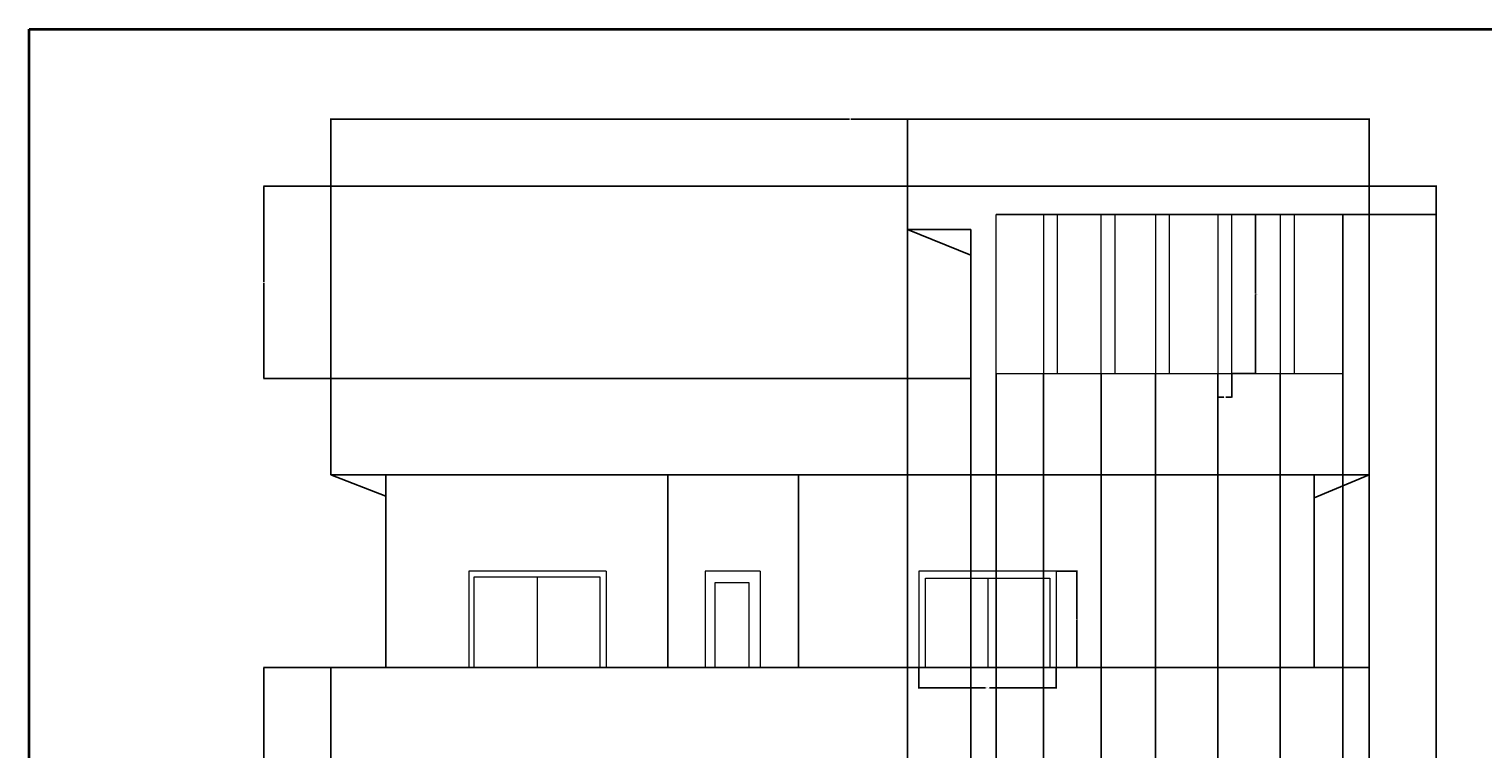
# Model space of a CAD drawing. Units: inches. Extents: x 1955 to 3324, y 980 to 3129.
# Tile 10 of 11: x 1955 to 2589, y 2815 to 3129. Entities that reach past the tile are written whole.
import ezdxf

# ---------------------------------------------------------------- set-up
doc = ezdxf.new("R2010")
doc.units = ezdxf.units.IN
for name, color, linetype, lineweight in [('A-ANNO-DIMS', 2, 'Continuous', 18), ('A-ANNO-TTLB', 7, 'Continuous', 35), ('A-ELEV', 7, 'Continuous', 25), ('A-GLAZ', 4, 'Continuous', 18), ('A-ROOF', 7, 'Continuous', 25)]:
    doc.layers.add(name, color=color, linetype=linetype, lineweight=lineweight)
doc.styles.get("Standard").update_dxf_attribs({"font": 'arial.ttf'})
doc.dimstyles.get("Standard").update_dxf_attribs({"dimtxt": 0.18, "dimasz": 0.18, "dimexe": 0.18, "dimexo": 0.0625, "dimgap": 0.09, "dimtad": 0, "dimtih": 1, "dimtoh": 1, "dimdec": 4, "dimzin": 0, "dimdsep": 46, "dimtxsty": 'Standard', "dimcen": 0.09, "dimadec": 0, "dimazin": 0, "dimtfac": 1, "dimtdec": 4, "dimtofl": 0, "dimtmove": 0, "dimatfit": 3, "dimfxl": 1, "dimtolj": 1, "dimtzin": 0, "dimarcsym": 0})

# ---------------------------------------------------------------- blocks, each defined once
blk = doc.blocks.new('WIN-ELEV-60-L')
for p, q in [((0, 42), (0, 0)), ((60, 42), (0, 42)), ((0, 42), (0, 0)), ((60, 42), (0, 42)), ((29.78, 39.43), (29.78, 0)), ((60, 42), (60, 0)), ((60, 42), (60, 0))]:
    blk.add_line(p, q)
blk.add_lwpolyline([(2.42, 0), (2.42, 39.43), (57.15, 39.43), (57.15, 0)])
blk = doc.blocks.new('WIN-ELEV-60-R')
for p, q in [((0, 42), (0, 0)), ((60, 42), (0, 42)), ((0, 42), (0, 0)), ((60, 42), (0, 42)), ((30.07, 38.91), (30.07, 0)), ((60, 42), (60, 0)), ((60, 42), (60, 0))]:
    blk.add_line(p, q)
blk.add_lwpolyline([(3, 0), (3, 38.91), (57.15, 38.91), (57.15, 0)])
blk = doc.blocks.new('WIN-ELEV-24')
for p, q in [((0, 42), (0, 0)), ((24, 42), (0, 42)), ((0, 42), (0, 0)), ((24, 42), (0, 42)), ((24, 42), (24, 0)), ((24, 42), (24, 0))]:
    blk.add_line(p, q)
blk.add_lwpolyline([(4.32, 0), (4.32, 37), (19.12, 37), (19.12, 0)])
blk = doc.blocks.new('SCREEN-MULLION')
for p, q in [((0, 69.3), (0, 0)), ((6.13, 0), (6.13, 69.3))]:
    blk.add_line(p, q)
blk = doc.blocks.new('*D51')
at = {"layer": 'A-ANNO-DIMS', "color": 0, "lineweight": -2, "transparency": 16777216}
for p, q in [((2479.31, 3047.98), (2489.82, 3047.98)), ((2489.64, 3047.8), (2489.64, 3013.51)), ((2489.64, 2978.85), (2489.64, 3013.14)), ((2479.31, 2978.67), (2489.82, 2978.67))]:
    blk.add_line(p, q, dxfattribs=at)
at = {"layer": 'A-ANNO-DIMS', "color": 0, "transparency": 16777216}
for points in [[(2489.61, 3047.8), (2489.67, 3047.8), (2489.64, 3047.98)], [(2489.61, 2978.85), (2489.67, 2978.85), (2489.64, 2978.67)]]:
    blk.add_solid(points, dxfattribs=at)
at = {"layer": 'Defpoints', "color": 0, "transparency": 16777216}
for p in [(2479.25, 3047.98), (2489.64, 3047.98), (2479.25, 2978.67)]:
    blk.add_point(p, dxfattribs=at)
at = {"layer": 'A-ANNO-DIMS', "color": 0, "transparency": 16777216, "insert": (2489.64, 3013.32), "char_height": 0.18, "attachment_point": 5}
blk.add_mtext('\\A1;MULLION 69 TYP.', dxfattribs=at)
blk = doc.blocks.new('*D52')
at = {"layer": 'A-ANNO-DIMS', "color": 0, "lineweight": -2, "transparency": 16777216}
for p, q in [((2473.12, 2978.61), (2473.12, 2968.1)), ((2479.25, 2978.61), (2479.25, 2968.1)), ((2473.3, 2968.28), (2475.72, 2968.28)), ((2479.07, 2968.28), (2476.64, 2968.28))]:
    blk.add_line(p, q, dxfattribs=at)
at = {"layer": 'A-ANNO-DIMS', "color": 0, "transparency": 16777216}
for points in [[(2473.3, 2968.31), (2473.3, 2968.25), (2473.12, 2968.28)], [(2479.07, 2968.31), (2479.07, 2968.25), (2479.25, 2968.28)]]:
    blk.add_solid(points, dxfattribs=at)
at = {"layer": 'Defpoints', "color": 0, "transparency": 16777216}
for p in [(2473.12, 2978.67), (2479.25, 2978.67), (2479.25, 2968.28)]:
    blk.add_point(p, dxfattribs=at)
at = {"layer": 'A-ANNO-DIMS', "color": 0, "transparency": 16777216, "insert": (2476.18, 2968.28), "char_height": 0.18, "attachment_point": 5}
blk.add_mtext('\\A1;6 TYP.', dxfattribs=at)
blk = doc.blocks.new('*D87')
at = {"layer": 'A-ANNO-DIMS', "color": 0, "lineweight": -2, "transparency": 16777216}
for p, q in [((2342.7, 2850.35), (2342.7, 2841.23)), ((2402.7, 2850.35), (2402.7, 2841.23)), ((2342.88, 2841.41), (2371.85, 2841.41)), ((2402.52, 2841.41), (2373.54, 2841.41))]:
    blk.add_line(p, q, dxfattribs=at)
at = {"layer": 'A-ANNO-DIMS', "color": 0, "transparency": 16777216}
for points in [[(2342.88, 2841.44), (2342.88, 2841.38), (2342.7, 2841.41)], [(2402.52, 2841.44), (2402.52, 2841.38), (2402.7, 2841.41)]]:
    blk.add_solid(points, dxfattribs=at)
at = {"layer": 'Defpoints', "color": 0, "transparency": 16777216}
for p in [(2342.7, 2850.41), (2402.7, 2850.41), (2402.7, 2841.41)]:
    blk.add_point(p, dxfattribs=at)
at = {"layer": 'A-ANNO-DIMS', "color": 0, "transparency": 16777216, "insert": (2372.7, 2841.41), "char_height": 0.18, "attachment_point": 5}
blk.add_mtext('\\A1;WIN. 60 TYP.', dxfattribs=at)
blk = doc.blocks.new('*D88')
at = {"layer": 'A-ANNO-DIMS', "color": 0, "lineweight": -2, "transparency": 16777216}
for p, q in [((2402.76, 2892.41), (2411.88, 2892.41)), ((2411.7, 2892.23), (2411.7, 2871.59)), ((2411.7, 2850.59), (2411.7, 2871.23)), ((2402.76, 2850.41), (2411.88, 2850.41))]:
    blk.add_line(p, q, dxfattribs=at)
at = {"layer": 'A-ANNO-DIMS', "color": 0, "transparency": 16777216}
for points in [[(2411.67, 2892.23), (2411.73, 2892.23), (2411.7, 2892.41)], [(2411.67, 2850.59), (2411.73, 2850.59), (2411.7, 2850.41)]]:
    blk.add_solid(points, dxfattribs=at)
at = {"layer": 'Defpoints', "color": 0, "transparency": 16777216}
for p in [(2402.7, 2892.41), (2411.7, 2892.41), (2402.7, 2850.41)]:
    blk.add_point(p, dxfattribs=at)
at = {"layer": 'A-ANNO-DIMS', "color": 0, "transparency": 16777216, "insert": (2411.7, 2871.41), "char_height": 0.18, "attachment_point": 5}
blk.add_mtext('\\A1;42 TYP.', dxfattribs=at)
blk = doc.blocks.new('*D112')
at = {"layer": 'A-ANNO-DIMS', "color": 0, "lineweight": -2, "transparency": 16777216}
for p, q in [((2086.21, 2976.47), (2086.21, 3089.84)), ((2086.39, 3089.66), (2312.42, 3089.66)), ((2539.03, 3089.66), (2313, 3089.66)), ((2539.21, 3060.47), (2539.21, 3089.84))]:
    blk.add_line(p, q, dxfattribs=at)
at = {"layer": 'A-ANNO-DIMS', "color": 0, "transparency": 16777216}
for points in [[(2086.39, 3089.69), (2086.39, 3089.63), (2086.21, 3089.66)], [(2539.03, 3089.69), (2539.03, 3089.63), (2539.21, 3089.66)]]:
    blk.add_solid(points, dxfattribs=at)
at = {"layer": 'Defpoints', "color": 0, "transparency": 16777216}
for p in [(2539.21, 3089.66), (2539.21, 3060.41), (2086.21, 2976.41)]:
    blk.add_point(p, dxfattribs=at)
at = {"layer": 'A-ANNO-DIMS', "color": 0, "transparency": 16777216, "insert": (2312.71, 3089.66), "char_height": 0.18, "attachment_point": 5}
blk.add_mtext('\\A1;453', dxfattribs=at)
blk = doc.blocks.new('*D113')
at = {"layer": 'A-ANNO-DIMS', "color": 0, "lineweight": -2, "transparency": 16777216}
for p, q in [((2539.27, 3060.41), (2568.64, 3060.41)), ((2568.46, 3060.23), (2568.46, 2799.59)), ((2568.46, 2538.59), (2568.46, 2799.23)), ((2539.27, 2538.41), (2568.64, 2538.41))]:
    blk.add_line(p, q, dxfattribs=at)
at = {"layer": 'A-ANNO-DIMS', "color": 0, "transparency": 16777216}
for points in [[(2568.43, 3060.23), (2568.49, 3060.23), (2568.46, 3060.41)], [(2568.43, 2538.59), (2568.49, 2538.59), (2568.46, 2538.41)]]:
    blk.add_solid(points, dxfattribs=at)
at = {"layer": 'Defpoints', "color": 0, "transparency": 16777216}
for p in [(2539.21, 3060.41), (2568.46, 3060.41), (2539.21, 2538.41)]:
    blk.add_point(p, dxfattribs=at)
at = {"layer": 'A-ANNO-DIMS', "color": 0, "transparency": 16777216, "insert": (2568.46, 2799.41), "char_height": 0.18, "attachment_point": 5}
blk.add_mtext('\\A1;522', dxfattribs=at)
blk = doc.blocks.new('*D120')
at = {"layer": 'A-ANNO-DIMS', "color": 0, "lineweight": -2, "transparency": 16777216}
for p, q in [((2086.15, 2850.41), (2056.78, 2850.41)), ((2056.96, 2850.23), (2056.96, 2787.59)), ((2056.96, 2724.59), (2056.96, 2787.23)), ((2086.15, 2724.41), (2056.78, 2724.41))]:
    blk.add_line(p, q, dxfattribs=at)
at = {"layer": 'A-ANNO-DIMS', "color": 0, "transparency": 16777216}
for points in [[(2056.93, 2850.23), (2056.99, 2850.23), (2056.96, 2850.41)], [(2056.93, 2724.59), (2056.99, 2724.59), (2056.96, 2724.41)]]:
    blk.add_solid(points, dxfattribs=at)
at = {"layer": 'Defpoints', "color": 0, "transparency": 16777216}
for p in [(2056.96, 2850.41), (2086.21, 2850.41), (2086.21, 2724.41)]:
    blk.add_point(p, dxfattribs=at)
at = {"layer": 'A-ANNO-DIMS', "color": 0, "transparency": 16777216, "insert": (2056.96, 2787.41), "char_height": 0.18, "attachment_point": 5}
blk.add_mtext('\\A1;126', dxfattribs=at)
blk = doc.blocks.new('*D121')
at = {"layer": 'A-ANNO-DIMS', "color": 0, "lineweight": -2, "transparency": 16777216}
for p, q in [((2337.71, 3060.41), (2056.78, 3060.41)), ((2056.96, 3060.23), (2056.96, 3018.59)), ((2056.96, 2976.59), (2056.96, 3018.23)), ((2365.4, 2976.41), (2056.78, 2976.41))]:
    blk.add_line(p, q, dxfattribs=at)
at = {"layer": 'A-ANNO-DIMS', "color": 0, "transparency": 16777216}
for points in [[(2056.93, 3060.23), (2056.99, 3060.23), (2056.96, 3060.41)], [(2056.93, 2976.59), (2056.99, 2976.59), (2056.96, 2976.41)]]:
    blk.add_solid(points, dxfattribs=at)
at = {"layer": 'Defpoints', "color": 0, "transparency": 16777216}
for p in [(2056.96, 3060.41), (2337.77, 3060.41), (2365.46, 2976.41)]:
    blk.add_point(p, dxfattribs=at)
at = {"layer": 'A-ANNO-DIMS', "color": 0, "transparency": 16777216, "insert": (2056.96, 3018.41), "char_height": 0.18, "attachment_point": 5}
blk.add_mtext('\\A1;84', dxfattribs=at)
blk = doc.blocks.new('*D122')
at = {"layer": 'A-ANNO-DIMS', "color": 0, "lineweight": -2, "transparency": 16777216}
for p, q in [((2337.77, 3060.47), (2337.77, 3089.84)), ((2337.95, 3089.66), (2438.03, 3089.66)), ((2539.03, 3089.66), (2438.95, 3089.66)), ((2539.21, 3060.47), (2539.21, 3089.84))]:
    blk.add_line(p, q, dxfattribs=at)
at = {"layer": 'A-ANNO-DIMS', "color": 0, "transparency": 16777216}
for points in [[(2337.95, 3089.69), (2337.95, 3089.63), (2337.77, 3089.66)], [(2539.03, 3089.69), (2539.03, 3089.63), (2539.21, 3089.66)]]:
    blk.add_solid(points, dxfattribs=at)
at = {"layer": 'Defpoints', "color": 0, "transparency": 16777216}
for p in [(2539.21, 3089.66), (2337.77, 3060.41), (2539.21, 3060.41)]:
    blk.add_point(p, dxfattribs=at)
at = {"layer": 'A-ANNO-DIMS', "color": 0, "transparency": 16777216, "insert": (2438.49, 3089.66), "char_height": 0.18, "attachment_point": 5}
blk.add_mtext('\\A1;201.44', dxfattribs=at)
blk = doc.blocks.new('*D123')
at = {"layer": 'A-ANNO-DIMS', "color": 0, "lineweight": -2, "transparency": 16777216}
for p, q in [((2337.77, 3041.34), (2337.77, 2454)), ((2365.46, 3041.34), (2365.46, 2454)), ((2337.95, 2454.18), (2351.22, 2454.18)), ((2365.28, 2454.18), (2352.01, 2454.18))]:
    blk.add_line(p, q, dxfattribs=at)
at = {"layer": 'A-ANNO-DIMS', "color": 0, "transparency": 16777216}
for points in [[(2337.95, 2454.21), (2337.95, 2454.15), (2337.77, 2454.18)], [(2365.28, 2454.21), (2365.28, 2454.15), (2365.46, 2454.18)]]:
    blk.add_solid(points, dxfattribs=at)
at = {"layer": 'Defpoints', "color": 0, "transparency": 16777216}
for p in [(2337.77, 3041.4), (2365.46, 3041.4), (2365.46, 2454.18)]:
    blk.add_point(p, dxfattribs=at)
at = {"layer": 'A-ANNO-DIMS', "color": 0, "transparency": 16777216, "insert": (2351.62, 2454.18), "char_height": 0.18, "attachment_point": 5}
blk.add_mtext('\\A1;27.69', dxfattribs=at)
blk = doc.blocks.new('*D124')
at = {"layer": 'A-ANNO-DIMS', "color": 0, "lineweight": -2, "transparency": 16777216}
for p, q in [((2376.45, 2978.61), (2376.45, 2454)), ((2397.08, 2978.61), (2397.08, 2454)), ((2376.63, 2454.18), (2386.37, 2454.18)), ((2396.9, 2454.18), (2387.16, 2454.18))]:
    blk.add_line(p, q, dxfattribs=at)
at = {"layer": 'A-ANNO-DIMS', "color": 0, "transparency": 16777216}
for points in [[(2376.63, 2454.21), (2376.63, 2454.15), (2376.45, 2454.18)], [(2396.9, 2454.21), (2396.9, 2454.15), (2397.08, 2454.18)]]:
    blk.add_solid(points, dxfattribs=at)
at = {"layer": 'Defpoints', "color": 0, "transparency": 16777216}
for p in [(2376.45, 2978.67), (2397.08, 2978.67), (2397.08, 2454.18)]:
    blk.add_point(p, dxfattribs=at)
at = {"layer": 'A-ANNO-DIMS', "color": 0, "transparency": 16777216, "insert": (2386.76, 2454.18), "char_height": 0.18, "attachment_point": 5}
blk.add_mtext('\\A1;20.63', dxfattribs=at)
blk = doc.blocks.new('*D125')
at = {"layer": 'A-ANNO-DIMS', "color": 0, "lineweight": -2, "transparency": 16777216}
for p, q in [((2397.08, 2978.61), (2397.08, 2454)), ((2422.2, 2978.61), (2422.2, 2454)), ((2397.26, 2454.18), (2409.24, 2454.18)), ((2422.02, 2454.18), (2410.03, 2454.18))]:
    blk.add_line(p, q, dxfattribs=at)
at = {"layer": 'A-ANNO-DIMS', "color": 0, "transparency": 16777216}
for points in [[(2397.26, 2454.21), (2397.26, 2454.15), (2397.08, 2454.18)], [(2422.02, 2454.21), (2422.02, 2454.15), (2422.2, 2454.18)]]:
    blk.add_solid(points, dxfattribs=at)
at = {"layer": 'Defpoints', "color": 0, "transparency": 16777216}
for p in [(2397.08, 2978.67), (2422.2, 2978.67), (2422.2, 2454.18)]:
    blk.add_point(p, dxfattribs=at)
at = {"layer": 'A-ANNO-DIMS', "color": 0, "transparency": 16777216, "insert": (2409.64, 2454.18), "char_height": 0.18, "attachment_point": 5}
blk.add_mtext('\\A1;25.12', dxfattribs=at)
blk = doc.blocks.new('*D126')
at = {"layer": 'A-ANNO-DIMS', "color": 0, "lineweight": -2, "transparency": 16777216}
for p, q in [((2422.2, 2978.61), (2422.2, 2454)), ((2445.92, 2978.61), (2445.92, 2454)), ((2422.38, 2454.18), (2433.59, 2454.18)), ((2445.74, 2454.18), (2434.52, 2454.18))]:
    blk.add_line(p, q, dxfattribs=at)
at = {"layer": 'A-ANNO-DIMS', "color": 0, "transparency": 16777216}
for points in [[(2422.38, 2454.21), (2422.38, 2454.15), (2422.2, 2454.18)], [(2445.74, 2454.21), (2445.74, 2454.15), (2445.92, 2454.18)]]:
    blk.add_solid(points, dxfattribs=at)
at = {"layer": 'Defpoints', "color": 0, "transparency": 16777216}
for p in [(2422.2, 2978.67), (2445.92, 2978.67), (2445.92, 2454.18)]:
    blk.add_point(p, dxfattribs=at)
at = {"layer": 'A-ANNO-DIMS', "color": 0, "transparency": 16777216, "insert": (2434.06, 2454.18), "char_height": 0.18, "attachment_point": 5}
blk.add_mtext('\\A1;23.727', dxfattribs=at)
blk = doc.blocks.new('*D127')
at = {"layer": 'A-ANNO-DIMS', "color": 0, "lineweight": -2, "transparency": 16777216}
for p, q in [((2445.92, 2978.61), (2445.92, 2454)), ((2473.12, 2978.61), (2473.12, 2454)), ((2446.1, 2454.18), (2459.05, 2454.18)), ((2472.94, 2454.18), (2459.99, 2454.18))]:
    blk.add_line(p, q, dxfattribs=at)
at = {"layer": 'A-ANNO-DIMS', "color": 0, "transparency": 16777216}
for points in [[(2446.1, 2454.21), (2446.1, 2454.15), (2445.92, 2454.18)], [(2472.94, 2454.21), (2472.94, 2454.15), (2473.12, 2454.18)]]:
    blk.add_solid(points, dxfattribs=at)
at = {"layer": 'Defpoints', "color": 0, "transparency": 16777216}
for p in [(2445.92, 2978.67), (2473.12, 2978.67), (2473.12, 2454.18)]:
    blk.add_point(p, dxfattribs=at)
at = {"layer": 'A-ANNO-DIMS', "color": 0, "transparency": 16777216, "insert": (2459.52, 2454.18), "char_height": 0.18, "attachment_point": 5}
blk.add_mtext('\\A1;27.195', dxfattribs=at)
blk = doc.blocks.new('*D128')
at = {"layer": 'A-ANNO-DIMS', "color": 0, "lineweight": -2, "transparency": 16777216}
for p, q in [((2473.12, 2978.61), (2473.12, 2454)), ((2500.43, 2978.61), (2500.43, 2454)), ((2473.3, 2454.18), (2486.31, 2454.18)), ((2500.25, 2454.18), (2487.24, 2454.18))]:
    blk.add_line(p, q, dxfattribs=at)
at = {"layer": 'A-ANNO-DIMS', "color": 0, "transparency": 16777216}
for points in [[(2473.3, 2454.21), (2473.3, 2454.15), (2473.12, 2454.18)], [(2500.25, 2454.21), (2500.25, 2454.15), (2500.43, 2454.18)]]:
    blk.add_solid(points, dxfattribs=at)
at = {"layer": 'Defpoints', "color": 0, "transparency": 16777216}
for p in [(2473.12, 2978.67), (2500.43, 2978.67), (2500.43, 2454.18)]:
    blk.add_point(p, dxfattribs=at)
at = {"layer": 'A-ANNO-DIMS', "color": 0, "transparency": 16777216, "insert": (2486.77, 2454.18), "char_height": 0.18, "attachment_point": 5}
blk.add_mtext('\\A1;27.314', dxfattribs=at)
blk = doc.blocks.new('*D129')
at = {"layer": 'A-ANNO-DIMS', "color": 0, "lineweight": -2, "transparency": 16777216}
for p, q in [((2500.43, 2978.61), (2500.43, 2454)), ((2527.66, 2978.61), (2527.66, 2454)), ((2500.61, 2454.18), (2513.65, 2454.18)), ((2527.48, 2454.18), (2514.44, 2454.18))]:
    blk.add_line(p, q, dxfattribs=at)
at = {"layer": 'A-ANNO-DIMS', "color": 0, "transparency": 16777216}
for points in [[(2500.61, 2454.21), (2500.61, 2454.15), (2500.43, 2454.18)], [(2527.48, 2454.21), (2527.48, 2454.15), (2527.66, 2454.18)]]:
    blk.add_solid(points, dxfattribs=at)
at = {"layer": 'Defpoints', "color": 0, "transparency": 16777216}
for p in [(2500.43, 2978.67), (2527.66, 2978.67), (2527.66, 2454.18)]:
    blk.add_point(p, dxfattribs=at)
at = {"layer": 'A-ANNO-DIMS', "color": 0, "transparency": 16777216, "insert": (2514.05, 2454.18), "char_height": 0.18, "attachment_point": 5}
blk.add_mtext('\\A1;27.23', dxfattribs=at)
blk = doc.blocks.new('*D130')
at = {"layer": 'A-ANNO-DIMS', "color": 0, "lineweight": -2, "transparency": 16777216}
for p, q in [((2539.21, 3060.35), (2539.21, 2454)), ((2527.66, 3047.91), (2527.66, 2454)), ((2527.84, 2454.18), (2533.05, 2454.18)), ((2539.03, 2454.18), (2533.82, 2454.18))]:
    blk.add_line(p, q, dxfattribs=at)
at = {"layer": 'A-ANNO-DIMS', "color": 0, "transparency": 16777216}
for points in [[(2527.84, 2454.21), (2527.84, 2454.15), (2527.66, 2454.18)], [(2539.03, 2454.21), (2539.03, 2454.15), (2539.21, 2454.18)]]:
    blk.add_solid(points, dxfattribs=at)
at = {"layer": 'Defpoints', "color": 0, "transparency": 16777216}
for p in [(2539.21, 3060.41), (2527.66, 3047.98), (2539.21, 2454.18)]:
    blk.add_point(p, dxfattribs=at)
at = {"layer": 'A-ANNO-DIMS', "color": 0, "transparency": 16777216, "insert": (2533.44, 2454.18), "char_height": 0.18, "attachment_point": 5}
blk.add_mtext('\\A1;11.55', dxfattribs=at)
blk = doc.blocks.new('*D131')
at = {"layer": 'A-ANNO-DIMS', "color": 0, "lineweight": -2, "transparency": 16777216}
for p, q in [((2337.83, 3060.41), (2568.64, 3060.41)), ((2568.46, 3060.23), (2568.46, 3054.37)), ((2568.46, 3048.16), (2568.46, 3054.01)), ((2376.51, 3047.98), (2568.64, 3047.98))]:
    blk.add_line(p, q, dxfattribs=at)
at = {"layer": 'A-ANNO-DIMS', "color": 0, "transparency": 16777216}
for points in [[(2568.43, 3060.23), (2568.49, 3060.23), (2568.46, 3060.41)], [(2568.43, 3048.16), (2568.49, 3048.16), (2568.46, 3047.98)]]:
    blk.add_solid(points, dxfattribs=at)
at = {"layer": 'Defpoints', "color": 0, "transparency": 16777216}
for p in [(2337.77, 3060.41), (2568.46, 3060.41), (2376.45, 3047.98)]:
    blk.add_point(p, dxfattribs=at)
at = {"layer": 'A-ANNO-DIMS', "color": 0, "transparency": 16777216, "insert": (2568.46, 3054.19), "char_height": 0.18, "attachment_point": 5}
blk.add_mtext('\\A1;12.435', dxfattribs=at)

msp = doc.modelspace()

# ---------------------------------------------------------------- linework, layer by layer
at = {"layer": 'A-ANNO-TTLB'}
msp.add_lwpolyline([(1954.5391, 3128.9103), (3323.9705, 3128.9103), (3323.9705, 1703.6826), (1954.5391, 1703.6826)], close=True, dxfattribs=at)
at = {"layer": 'A-ELEV'}
for p, q in [((2365.4619, 2976.4103), (2086.2102, 2976.4103)), ((2086.2102, 2934.4103), (2086.2102, 2976.4103)), ((2539.2102, 2934.4103), (2539.2102, 2976.4103)), ((2539.2102, 2934.4103), (2086.2102, 2934.4103)), ((2086.2102, 2934.4103), (2110.2102, 2925.0754)), ((2110.2102, 2934.4103), (2110.2102, 2850.4103)), ((2233.2102, 2934.4103), (2233.2102, 2850.4103)), ((2290.2102, 2934.4103), (2290.2102, 2850.4103)), ((2515.2102, 2934.4103), (2515.2102, 2850.4103)), ((2539.2102, 2934.4103), (2515.2102, 2924.3558)), ((2539.2102, 2850.4103), (2086.2102, 2850.4103)), ((2086.2102, 2808.4103), (2086.2102, 2850.4103)), ((2539.2102, 2808.4103), (2539.2102, 2850.4103))]:
    msp.add_line(p, q, dxfattribs=at)
at = {"layer": 'A-GLAZ'}
msp.add_line((2376.4478, 2978.6742), (2527.661, 2978.6742), dxfattribs=at)
msp.add_lwpolyline([(2376.4478, 2978.6742), (2376.4478, 3047.9754), (2527.661, 3047.9754), (2527.661, 2978.6742)], dxfattribs=at)
at = {"layer": 'A-ROOF'}
for p, q in [((2365.4619, 3060.4103), (2337.7695, 3060.4103)), ((2337.7695, 3060.4103), (2337.7695, 3041.4019)), ((2539.2102, 3060.4103), (2365.4619, 3060.4103)), ((2539.2102, 2976.4103), (2539.2102, 3060.4103)), ((2337.7695, 3041.4019), (2365.4619, 3041.4019)), ((2337.7695, 3041.4019), (2365.4619, 3030.2391)), ((2365.4619, 3041.4019), (2365.4619, 2976.4103))]:
    msp.add_line(p, q, dxfattribs=at)

# ---------------------------------------------------------------- block references
at = {"layer": 'A-GLAZ'}
for name, p in [('SCREEN-MULLION', (2397.077, 2978.674)), ('SCREEN-MULLION', (2422.1948, 2978.674)), ('SCREEN-MULLION', (2445.922, 2978.674)), ('SCREEN-MULLION', (2473.1166, 2978.674)), ('SCREEN-MULLION', (2500.4304, 2978.674)), ('WIN-ELEV-60-L', (2146.362, 2850.41)), ('WIN-ELEV-24', (2249.489, 2850.41)), ('WIN-ELEV-60-R', (2342.696, 2850.41))]:
    msp.add_blockref(name, p, dxfattribs=at)

# ---------------------------------------------------------------- dimensions: what is measured, and where the dimension line sits
at = {"layer": 'A-ANNO-DIMS'}
for base, p1, p2, override, picture, middle in [((2539.2102, 3089.6603), (2086.2102, 2976.4103), (2539.2102, 3060.4103), {"dimdec": 0, "dimlfac": 1, "dimrnd": 0, "dimzin": 0, "dimdsep": 46, "dimlunit": 2}, '*D112', (2312.7102, 3089.6603)), ((2539.2102, 3089.6603), (2337.7695, 3060.4103), (2539.2102, 3060.4103), {"dimdec": 2, "dimlfac": 1, "dimrnd": 0, "dimzin": 0, "dimdsep": 46, "dimlunit": 2}, '*D122', (2438.4899, 3089.6603)), ((2539.2102, 2454.185), (2527.661, 3047.9754), (2539.2102, 3060.4103), {"dimdec": 2, "dimlfac": 1, "dimrnd": 0, "dimzin": 0, "dimdsep": 46, "dimlunit": 2}, '*D130', (2533.4356, 2454.185)), ((2365.4619, 2454.185), (2337.7695, 3041.4019), (2365.4619, 3041.4019), {"dimdec": 2, "dimlfac": 1, "dimrnd": 0, "dimzin": 0, "dimdsep": 46, "dimlunit": 2}, '*D123', (2351.6157, 2454.185)), ((2397.0773, 2454.185), (2376.4478, 2978.6742), (2397.0773, 2978.6742), {"dimdec": 2, "dimlfac": 1, "dimrnd": 0, "dimzin": 0, "dimdsep": 46, "dimlunit": 2}, '*D124', (2386.7626, 2454.185)), ((2422.1951, 2454.185), (2397.0773, 2978.6742), (2422.1951, 2978.6742), {"dimdec": 2, "dimlfac": 1, "dimrnd": 0, "dimzin": 0, "dimdsep": 46, "dimlunit": 2}, '*D125', (2409.6362, 2454.185)), ((2445.9223, 2454.185), (2422.1951, 2978.6742), (2445.9223, 2978.6742), {"dimdec": 3, "dimlfac": 1, "dimrnd": 0, "dimzin": 0, "dimdsep": 46, "dimlunit": 2}, '*D126', (2434.0587, 2454.185)), ((2473.1169, 2454.185), (2445.9223, 2978.6742), (2473.1169, 2978.6742), {"dimdec": 3, "dimlfac": 1, "dimrnd": 0, "dimzin": 0, "dimdsep": 46, "dimlunit": 2}, '*D127', (2459.5196, 2454.185)), ((2500.4308, 2454.185), (2473.1169, 2978.6742), (2500.4308, 2978.6742), {"dimdec": 3, "dimlfac": 1, "dimrnd": 0, "dimzin": 0, "dimdsep": 46, "dimlunit": 2}, '*D128', (2486.7738, 2454.185)), ((2527.661, 2454.185), (2500.4308, 2978.6742), (2527.661, 2978.6742), {"dimdec": 2, "dimlfac": 1, "dimrnd": 0, "dimzin": 0, "dimdsep": 46, "dimlunit": 2}, '*D129', (2514.0459, 2454.185))]:
    dim = msp.add_linear_dim(base=base, p1=p1, p2=p2, dimstyle='Standard', override=override, dxfattribs=at)
    dim.commit()
    dim.dimension.update_dxf_attribs({"geometry": picture, "text_midpoint": middle})
for base, p1, p2, override, picture, middle in [((2056.9602, 3060.4103), (2365.4619, 2976.4103), (2337.7695, 3060.4103), {"dimdec": 0, "dimlfac": 1, "dimrnd": 0, "dimzin": 0, "dimdsep": 46, "dimlunit": 2}, '*D121', (2056.9602, 3018.4103)), ((2568.4602, 3060.4103), (2376.4478, 3047.9754), (2337.7695, 3060.4103), {"dimdec": 3, "dimlfac": 1, "dimrnd": 0, "dimzin": 0, "dimdsep": 46, "dimlunit": 2}, '*D131', (2568.4602, 3054.1928)), ((2568.4602, 3060.4103), (2539.2102, 2538.4103), (2539.2102, 3060.4103), {"dimdec": 0, "dimlfac": 1, "dimrnd": 0, "dimzin": 0, "dimdsep": 46, "dimlunit": 2}, '*D113', (2568.4602, 2799.4103)), ((2056.9602, 2850.4103), (2086.2102, 2724.4103), (2086.2102, 2850.4103), {"dimdec": 0, "dimlfac": 1, "dimrnd": 0, "dimzin": 0, "dimdsep": 46, "dimlunit": 2}, '*D120', (2056.9602, 2787.4103))]:
    dim = msp.add_linear_dim(base=base, p1=p1, p2=p2, angle=90, dimstyle='Standard', override=override, dxfattribs=at)
    dim.commit()
    dim.dimension.update_dxf_attribs({"geometry": picture, "text_midpoint": middle})
for base, p1, p2, text, picture, middle in [((2489.6441, 3047.9754), (2479.249, 2978.6742), (2479.249, 3047.9754), 'MULLION <> TYP.', '*D51', (2489.6441, 3013.3248)), ((2411.6963, 2892.4103), (2402.6963, 2850.4103), (2402.6963, 2892.4103), '<> TYP.', '*D88', (2411.6963, 2871.4103))]:
    dim = msp.add_linear_dim(base=base, p1=p1, p2=p2, angle=90, text=text, dimstyle='Standard', override={"dimdec": 0, "dimlfac": 1, "dimrnd": 0, "dimzin": 0, "dimdsep": 46, "dimlunit": 2}, dxfattribs=at)
    dim.commit()
    dim.dimension.update_dxf_attribs({"geometry": picture, "text_midpoint": middle})
for base, p1, p2, text, picture, middle in [((2479.249, 2968.279), (2473.1169, 2978.6742), (2479.249, 2978.6742), '<> TYP.', '*D52', (2476.1829, 2968.279)), ((2402.6963, 2841.4103), (2342.6963, 2850.4103), (2402.6963, 2850.4103), 'WIN. <> TYP.', '*D87', (2372.6963, 2841.4103))]:
    dim = msp.add_linear_dim(base=base, p1=p1, p2=p2, text=text, dimstyle='Standard', override={"dimdec": 0, "dimlfac": 1, "dimrnd": 0, "dimzin": 0, "dimdsep": 46, "dimlunit": 2}, dxfattribs=at)
    dim.commit()
    dim.dimension.update_dxf_attribs({"geometry": picture, "text_midpoint": middle})

doc.saveas('drawing.dxf')
